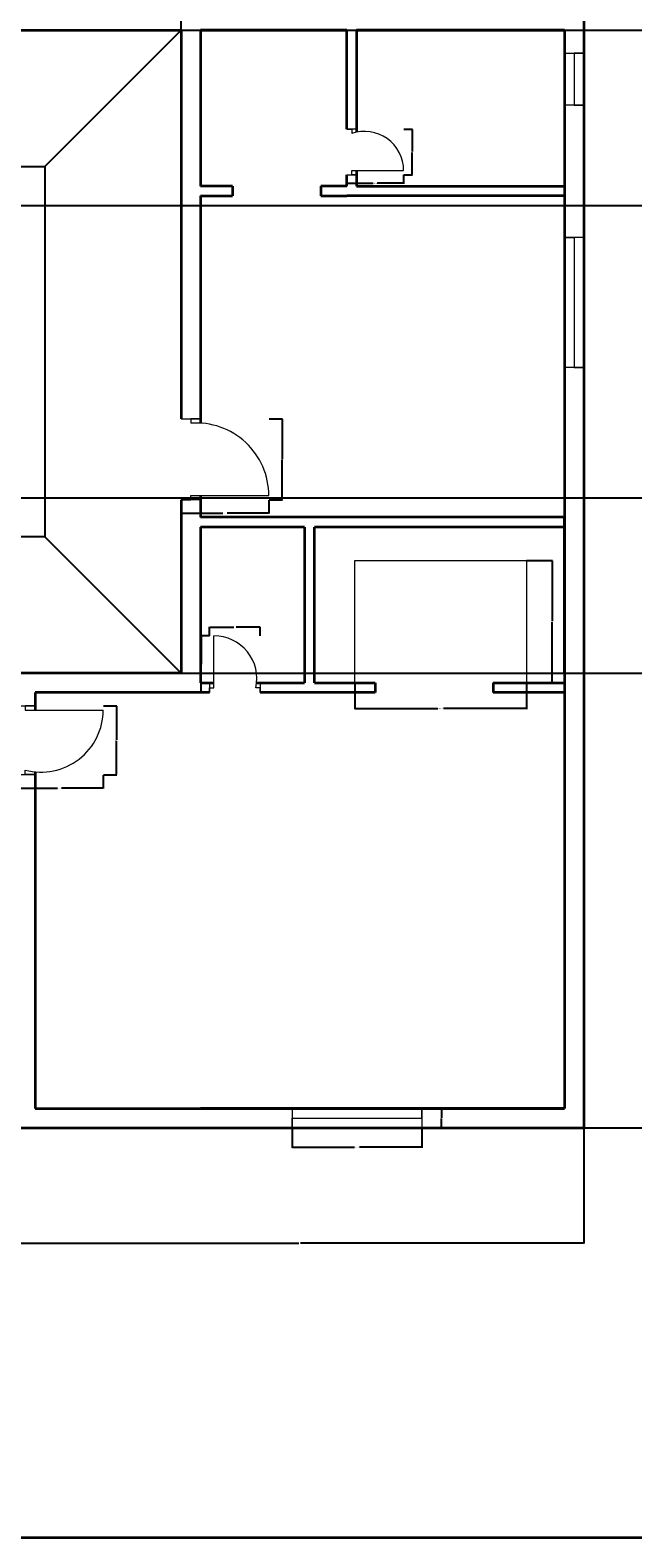
# Model space of a CAD drawing. Units: inches. Extents: x 2185 to 4426, y 1138 to 3073.
# Tile 10 of 14: x 3677 to 3955, y 1138 to 1834. Entities that reach past the tile are written whole.
import ezdxf

# ---------------------------------------------------------------- set-up
doc = ezdxf.new("R2010")
doc.units = ezdxf.units.IN
for name, color, linetype, lineweight in [('A-ANNO-DIMS', 2, 'Continuous', 18), ('A-ANNO-TTLB', 7, 'Continuous', 35), ('A-DOOR', 3, 'Continuous', 18), ('A-FLOR-CASE', 32, 'Continuous', 18), ('A-FLOR-EDGE', 7, 'Continuous', 25), ('A-GLAZ', 4, 'Continuous', 18), ('A-WALL', 7, 'Continuous', 35)]:
    doc.layers.add(name, color=color, linetype=linetype, lineweight=lineweight)
doc.styles.get("Standard").update_dxf_attribs({"font": 'arial.ttf'})
doc.dimstyles.get("Standard").update_dxf_attribs({"dimtxt": 0.18, "dimasz": 0.18, "dimexe": 0.18, "dimexo": 0.0625, "dimgap": 0.09, "dimtad": 0, "dimtih": 1, "dimtoh": 1, "dimdec": 4, "dimzin": 0, "dimdsep": 46, "dimtxsty": 'Standard', "dimcen": 0.09, "dimadec": 0, "dimazin": 0, "dimtfac": 1, "dimtdec": 4, "dimtofl": 0, "dimtmove": 0, "dimatfit": 3, "dimfxl": 1, "dimtolj": 1, "dimtzin": 0, "dimarcsym": 0})

# ---------------------------------------------------------------- blocks, each defined once
blk = doc.blocks.new('DOOR-SGL-24-BATH-S')
for p, q in [((2, 2.25), (2, 26.25)), ((0, 4.5), (0, 0)), ((0, 0), (0, 2.25)), ((0, 2.25), (0, 2.25)), ((0, 2.25), (2, 2.25)), ((23.36, 2.25), (21.36, 2.25)), ((23.36, 4.5), (23.36, 4.5)), ((23.36, 4.5), (23.36, 0)), ((23.36, 0), (23.36, 2.25))]:
    blk.add_line(p, q)
blk.add_arc((2, 6.44), 19.81, 347.78651, 90)
blk = doc.blocks.new('DOOR-SGL-36-BED-SE')
for p, q in [((0, 37.45), (9, 37.45)), ((9, 37.45), (4.5, 37.45)), ((4.5, 37.45), (4.5, 35.45)), ((9, 0), (0, 0)), ((0, 0), (4.5, 0)), ((4.5, 0), (4.5, 2)), ((4.5, 2), (40.5, 2))]:
    blk.add_line(p, q)
blk.add_arc((6.96, 2), 33.54, 0, 94.21362)
blk = doc.blocks.new('DOOR-SGL-24-BATH-E')
for p, q in [((4.5, 21.05), (0, 21.05)), ((0, 21.05), (2.25, 21.05)), ((2.25, 21.05), (2.25, 19.05)), ((0, 0), (4.5, 0)), ((2.25, 0), (2.25, 2)), ((2.25, 2), (26.25, 2)), ((4.5, 0), (2.25, 0))]:
    blk.add_line(p, q)
blk.add_arc((8.19, 2), 18.06, 0, 109.21567)
blk = doc.blocks.new('DOOR-SGL-36-BED-S')
for p, q in [((0, 31.73), (9, 31.73)), ((9, 31.73), (4.5, 31.73)), ((4.5, 31.73), (4.5, 31.73)), ((4.5, 31.73), (4.5, 29.73)), ((4.5, 29.73), (40.5, 29.73)), ((0, 0), (9, 0)), ((4.5, 0), (4.5, 2)), ((9, 0), (4.5, 0))]:
    blk.add_line(p, q)
blk.add_arc((11.82, 29.73), 28.68, 255.21093, 0)
blk = doc.blocks.new('WIN-PLAN-24IN-03')
for p, q in [((0, 24), (9, 24)), ((9, 24), (4.5, 24)), ((4.5, 24), (4.5, 0)), ((9, 0), (0, 0)), ((4.5, 0), (9, 0))]:
    blk.add_line(p, q)
blk = doc.blocks.new('WIN-PLAN-60IN-01')
for p, q in [((0, 9), (0, 0)), ((60, 4.5), (60, 9)), ((60, 9), (60, 0)), ((0, 0), (0, 4.5)), ((0, 4.5), (0, 4.5)), ((0, 4.5), (60, 4.5))]:
    blk.add_line(p, q)
blk = doc.blocks.new('WARDROBE-U')
for p, q in [((0, 0), (0, 56.6)), ((0, 56.6), (79.32, 56.6)), ((79.32, 56.6), (79.32, 0))]:
    blk.add_line(p, q)
blk = doc.blocks.new('*D60')
at = {"layer": 'A-ANNO-DIMS', "color": 0, "lineweight": -2, "transparency": 16777216}
for p, q in [((3797.54, 1327.31), (3797.54, 1318.2)), ((3857.54, 1327.31), (3857.54, 1318.2)), ((3797.72, 1318.38), (3826.42, 1318.38)), ((3857.36, 1318.38), (3828.66, 1318.38))]:
    blk.add_line(p, q, dxfattribs=at)
at = {"layer": 'A-ANNO-DIMS', "color": 0, "transparency": 16777216}
for points in [[(3797.72, 1318.41), (3797.72, 1318.35), (3797.54, 1318.38)], [(3857.36, 1318.41), (3857.36, 1318.35), (3857.54, 1318.38)]]:
    blk.add_solid(points, dxfattribs=at)
at = {"layer": 'Defpoints', "color": 0, "transparency": 16777216}
for p in [(3797.54, 1327.38), (3857.54, 1327.38), (3857.54, 1318.38)]:
    blk.add_point(p, dxfattribs=at)
at = {"layer": 'A-ANNO-DIMS', "color": 0, "transparency": 16777216, "insert": (3827.54, 1318.38), "char_height": 0.18, "attachment_point": 5}
blk.add_mtext('\\A1;WINDOW 60 TYP.', dxfattribs=at)
blk = doc.blocks.new('*D61')
at = {"layer": 'A-ANNO-DIMS', "color": 0, "lineweight": -2, "transparency": 16777216}
for p, q in [((3857.6, 1336.38), (3866.72, 1336.38)), ((3866.54, 1336.2), (3866.54, 1332.06)), ((3866.54, 1327.56), (3866.54, 1331.7)), ((3857.6, 1327.38), (3866.72, 1327.38))]:
    blk.add_line(p, q, dxfattribs=at)
at = {"layer": 'A-ANNO-DIMS', "color": 0, "transparency": 16777216}
for points in [[(3866.51, 1336.2), (3866.57, 1336.2), (3866.54, 1336.38)], [(3866.51, 1327.56), (3866.57, 1327.56), (3866.54, 1327.38)]]:
    blk.add_solid(points, dxfattribs=at)
at = {"layer": 'Defpoints', "color": 0, "transparency": 16777216}
for p in [(3857.54, 1336.38), (3866.54, 1336.38), (3857.54, 1327.38)]:
    blk.add_point(p, dxfattribs=at)
at = {"layer": 'A-ANNO-DIMS', "color": 0, "transparency": 16777216, "insert": (3866.54, 1331.88), "char_height": 0.18, "attachment_point": 5}
blk.add_mtext('\\A1;9 TYP.', dxfattribs=at)
blk = doc.blocks.new('*D78')
at = {"layer": 'A-ANNO-DIMS', "color": 0, "lineweight": -2, "transparency": 16777216}
for p, q in [((3759.43, 1554.63), (3755.38, 1554.63)), ((3755.56, 1554.45), (3755.56, 1541.69)), ((3755.56, 1528.56), (3755.56, 1541.32)), ((3759.43, 1528.38), (3755.38, 1528.38))]:
    blk.add_line(p, q, dxfattribs=at)
at = {"layer": 'A-ANNO-DIMS', "color": 0, "transparency": 16777216}
for points in [[(3755.53, 1554.45), (3755.59, 1554.45), (3755.56, 1554.63)], [(3755.53, 1528.56), (3755.59, 1528.56), (3755.56, 1528.38)]]:
    blk.add_solid(points, dxfattribs=at)
at = {"layer": 'Defpoints', "color": 0, "transparency": 16777216}
for p in [(3755.56, 1554.63), (3759.5, 1554.63), (3759.5, 1528.38)]:
    blk.add_point(p, dxfattribs=at)
at = {"layer": 'A-ANNO-DIMS', "color": 0, "transparency": 16777216, "insert": (3755.56, 1541.5), "char_height": 0.18, "attachment_point": 5}
blk.add_mtext('\\A1;DOOR 26 TYP.', dxfattribs=at)
blk = doc.blocks.new('*D79')
at = {"layer": 'A-ANNO-DIMS', "color": 0, "lineweight": -2, "transparency": 16777216}
for p, q in [((3759.5, 1554.69), (3759.5, 1558.74)), ((3759.68, 1558.56), (3770.65, 1558.56)), ((3782.68, 1558.56), (3771.71, 1558.56)), ((3782.86, 1554.69), (3782.86, 1558.74))]:
    blk.add_line(p, q, dxfattribs=at)
at = {"layer": 'A-ANNO-DIMS', "color": 0, "transparency": 16777216}
for points in [[(3759.68, 1558.59), (3759.68, 1558.53), (3759.5, 1558.56)], [(3782.68, 1558.59), (3782.68, 1558.53), (3782.86, 1558.56)]]:
    blk.add_solid(points, dxfattribs=at)
at = {"layer": 'Defpoints', "color": 0, "transparency": 16777216}
for p in [(3759.5, 1554.63), (3782.86, 1558.56), (3782.86, 1554.63)]:
    blk.add_point(p, dxfattribs=at)
at = {"layer": 'A-ANNO-DIMS', "color": 0, "transparency": 16777216, "insert": (3771.18, 1558.56), "char_height": 0.18, "attachment_point": 5}
blk.add_mtext('\\A1;23 TYP.', dxfattribs=at)
blk = doc.blocks.new('*D82')
at = {"layer": 'A-ANNO-DIMS', "color": 0, "lineweight": -2, "transparency": 16777216}
for p, q in [((3746.35, 1617.31), (3746.35, 1611.12)), ((3786.85, 1617.31), (3786.85, 1611.12)), ((3746.53, 1611.3), (3765.66, 1611.3)), ((3786.67, 1611.3), (3767.53, 1611.3))]:
    blk.add_line(p, q, dxfattribs=at)
at = {"layer": 'A-ANNO-DIMS', "color": 0, "transparency": 16777216}
for points in [[(3746.53, 1611.33), (3746.53, 1611.27), (3746.35, 1611.3)], [(3786.67, 1611.33), (3786.67, 1611.27), (3786.85, 1611.3)]]:
    blk.add_solid(points, dxfattribs=at)
at = {"layer": 'Defpoints', "color": 0, "transparency": 16777216}
for p in [(3746.35, 1617.38), (3786.85, 1617.38), (3786.85, 1611.3)]:
    blk.add_point(p, dxfattribs=at)
at = {"layer": 'A-ANNO-DIMS', "color": 0, "transparency": 16777216, "insert": (3766.6, 1611.3), "char_height": 0.18, "attachment_point": 5}
blk.add_mtext('\\A1;DOOR 41 TYP.', dxfattribs=at)
blk = doc.blocks.new('*D83')
at = {"layer": 'A-ANNO-DIMS', "color": 0, "lineweight": -2, "transparency": 16777216}
for p, q in [((3786.91, 1654.82), (3793.1, 1654.82)), ((3792.92, 1654.64), (3792.92, 1636.28)), ((3792.92, 1617.56), (3792.92, 1635.92)), ((3786.91, 1617.38), (3793.1, 1617.38))]:
    blk.add_line(p, q, dxfattribs=at)
at = {"layer": 'A-ANNO-DIMS', "color": 0, "transparency": 16777216}
for points in [[(3792.89, 1654.64), (3792.95, 1654.64), (3792.92, 1654.82)], [(3792.89, 1617.56), (3792.95, 1617.56), (3792.92, 1617.38)]]:
    blk.add_solid(points, dxfattribs=at)
at = {"layer": 'Defpoints', "color": 0, "transparency": 16777216}
for p in [(3786.85, 1654.82), (3792.92, 1654.82), (3786.85, 1617.38)]:
    blk.add_point(p, dxfattribs=at)
at = {"layer": 'A-ANNO-DIMS', "color": 0, "transparency": 16777216, "insert": (3792.92, 1636.1), "char_height": 0.18, "attachment_point": 5}
blk.add_mtext('\\A1;37 TYP.', dxfattribs=at)
blk = doc.blocks.new('*D84')
at = {"layer": 'A-ANNO-DIMS', "color": 0, "lineweight": -2, "transparency": 16777216}
for p, q in [((3822.85, 1767.5), (3822.85, 1763.45)), ((3823.03, 1763.63), (3835.04, 1763.63)), ((3848.92, 1763.63), (3836.91, 1763.63)), ((3849.1, 1767.5), (3849.1, 1763.45))]:
    blk.add_line(p, q, dxfattribs=at)
at = {"layer": 'A-ANNO-DIMS', "color": 0, "transparency": 16777216}
for points in [[(3823.03, 1763.66), (3823.03, 1763.6), (3822.85, 1763.63)], [(3848.92, 1763.66), (3848.92, 1763.6), (3849.1, 1763.63)]]:
    blk.add_solid(points, dxfattribs=at)
at = {"layer": 'Defpoints', "color": 0, "transparency": 16777216}
for p in [(3822.85, 1767.56), (3849.1, 1767.56), (3849.1, 1763.63)]:
    blk.add_point(p, dxfattribs=at)
at = {"layer": 'A-ANNO-DIMS', "color": 0, "transparency": 16777216, "insert": (3835.97, 1763.63), "char_height": 0.18, "attachment_point": 5}
blk.add_mtext('\\A1;DOOR 26 TYP.', dxfattribs=at)
blk = doc.blocks.new('*D85')
at = {"layer": 'A-ANNO-DIMS', "color": 0, "lineweight": -2, "transparency": 16777216}
for p, q in [((3849.16, 1788.61), (3853.22, 1788.61)), ((3853.04, 1788.43), (3853.04, 1778.27)), ((3853.04, 1767.74), (3853.04, 1777.91)), ((3849.16, 1767.56), (3853.22, 1767.56))]:
    blk.add_line(p, q, dxfattribs=at)
at = {"layer": 'A-ANNO-DIMS', "color": 0, "transparency": 16777216}
for points in [[(3853.01, 1788.43), (3853.07, 1788.43), (3853.04, 1788.61)], [(3853.01, 1767.74), (3853.07, 1767.74), (3853.04, 1767.56)]]:
    blk.add_solid(points, dxfattribs=at)
at = {"layer": 'Defpoints', "color": 0, "transparency": 16777216}
for p in [(3849.1, 1788.61), (3853.04, 1788.61), (3849.1, 1767.56)]:
    blk.add_point(p, dxfattribs=at)
at = {"layer": 'A-ANNO-DIMS', "color": 0, "transparency": 16777216, "insert": (3853.04, 1778.09), "char_height": 0.18, "attachment_point": 5}
blk.add_mtext('\\A1;21 TYP.', dxfattribs=at)
blk = doc.blocks.new('*D90')
at = {"layer": 'A-ANNO-DIMS', "color": 0, "lineweight": -2, "transparency": 16777216}
for p, q in [((3669.85, 1490.29), (3669.85, 1484.1)), ((3710.35, 1490.29), (3710.35, 1484.1)), ((3670.03, 1484.28), (3689.16, 1484.28)), ((3710.17, 1484.28), (3691.03, 1484.28))]:
    blk.add_line(p, q, dxfattribs=at)
at = {"layer": 'A-ANNO-DIMS', "color": 0, "transparency": 16777216}
for points in [[(3670.03, 1484.31), (3670.03, 1484.25), (3669.85, 1484.28)], [(3710.17, 1484.31), (3710.17, 1484.25), (3710.35, 1484.28)]]:
    blk.add_solid(points, dxfattribs=at)
at = {"layer": 'Defpoints', "color": 0, "transparency": 16777216}
for p in [(3669.85, 1490.36), (3710.35, 1490.36), (3710.35, 1484.28)]:
    blk.add_point(p, dxfattribs=at)
at = {"layer": 'A-ANNO-DIMS', "color": 0, "transparency": 16777216, "insert": (3690.1, 1484.28), "char_height": 0.18, "attachment_point": 5}
blk.add_mtext('\\A1;DOOR 41 TYP.', dxfattribs=at)
blk = doc.blocks.new('*D91')
at = {"layer": 'A-ANNO-DIMS', "color": 0, "lineweight": -2, "transparency": 16777216}
for p, q in [((3710.41, 1522.36), (3716.6, 1522.36)), ((3716.42, 1522.18), (3716.42, 1506.54)), ((3716.42, 1490.54), (3716.42, 1506.17)), ((3710.41, 1490.36), (3716.6, 1490.36))]:
    blk.add_line(p, q, dxfattribs=at)
at = {"layer": 'A-ANNO-DIMS', "color": 0, "transparency": 16777216}
for points in [[(3716.39, 1522.18), (3716.45, 1522.18), (3716.42, 1522.36)], [(3716.39, 1490.54), (3716.45, 1490.54), (3716.42, 1490.36)]]:
    blk.add_solid(points, dxfattribs=at)
at = {"layer": 'Defpoints', "color": 0, "transparency": 16777216}
for p in [(3710.35, 1522.36), (3716.42, 1522.36), (3710.35, 1490.36)]:
    blk.add_point(p, dxfattribs=at)
at = {"layer": 'A-ANNO-DIMS', "color": 0, "transparency": 16777216, "insert": (3716.42, 1506.36), "char_height": 0.18, "attachment_point": 5}
blk.add_mtext('\\A1;32 TYP.', dxfattribs=at)
blk = doc.blocks.new('*D122')
at = {"layer": 'A-ANNO-DIMS', "color": 0, "lineweight": -2, "transparency": 16777216}
for p, q in [((3826.51, 1532.81), (3826.51, 1520.8)), ((3905.83, 1532.81), (3905.83, 1520.8)), ((3826.69, 1520.98), (3864.86, 1520.98)), ((3905.65, 1520.98), (3867.48, 1520.98))]:
    blk.add_line(p, q, dxfattribs=at)
at = {"layer": 'A-ANNO-DIMS', "color": 0, "transparency": 16777216}
for points in [[(3826.69, 1521.01), (3826.69, 1520.95), (3826.51, 1520.98)], [(3905.65, 1521.01), (3905.65, 1520.95), (3905.83, 1520.98)]]:
    blk.add_solid(points, dxfattribs=at)
at = {"layer": 'Defpoints', "color": 0, "transparency": 16777216}
for p in [(3826.51, 1532.88), (3905.83, 1532.88), (3905.83, 1520.98)]:
    blk.add_point(p, dxfattribs=at)
at = {"layer": 'A-ANNO-DIMS', "color": 0, "transparency": 16777216, "insert": (3866.17, 1520.98), "char_height": 0.18, "attachment_point": 5}
blk.add_mtext('\\A1;WARDROBE 79 TYP.', dxfattribs=at)
blk = doc.blocks.new('*D123')
at = {"layer": 'A-ANNO-DIMS', "color": 0, "lineweight": -2, "transparency": 16777216}
for p, q in [((3905.89, 1589.48), (3917.91, 1589.48)), ((3917.73, 1589.3), (3917.73, 1561.36)), ((3917.73, 1533.06), (3917.73, 1561)), ((3905.89, 1532.88), (3917.91, 1532.88))]:
    blk.add_line(p, q, dxfattribs=at)
at = {"layer": 'A-ANNO-DIMS', "color": 0, "transparency": 16777216}
for points in [[(3917.7, 1589.3), (3917.76, 1589.3), (3917.73, 1589.48)], [(3917.7, 1533.06), (3917.76, 1533.06), (3917.73, 1532.88)]]:
    blk.add_solid(points, dxfattribs=at)
at = {"layer": 'Defpoints', "color": 0, "transparency": 16777216}
for p in [(3905.83, 1589.48), (3917.73, 1589.48), (3905.83, 1532.88)]:
    blk.add_point(p, dxfattribs=at)
at = {"layer": 'A-ANNO-DIMS', "color": 0, "transparency": 16777216, "insert": (3917.73, 1561.18), "char_height": 0.18, "attachment_point": 5}
blk.add_mtext('\\A1;57 TYP.', dxfattribs=at)
blk = doc.blocks.new('*D146')
at = {"layer": 'A-ANNO-DIMS', "color": 0, "lineweight": -2, "transparency": 16777216}
for p, q in [((3932.41, 2326.38), (4058.64, 2326.38)), ((4058.46, 2326.2), (4058.46, 1827.06)), ((4058.46, 1327.56), (4058.46, 1826.7)), ((3932.41, 1327.38), (4058.64, 1327.38))]:
    blk.add_line(p, q, dxfattribs=at)
at = {"layer": 'A-ANNO-DIMS', "color": 0, "transparency": 16777216}
for points in [[(4058.43, 2326.2), (4058.49, 2326.2), (4058.46, 2326.38)], [(4058.43, 1327.56), (4058.49, 1327.56), (4058.46, 1327.38)]]:
    blk.add_solid(points, dxfattribs=at)
at = {"layer": 'Defpoints', "color": 0, "transparency": 16777216}
for p in [(3932.35, 2326.38), (4058.46, 2326.38), (3932.35, 1327.38)]:
    blk.add_point(p, dxfattribs=at)
at = {"layer": 'A-ANNO-DIMS', "color": 0, "transparency": 16777216, "insert": (4058.46, 1826.88), "char_height": 0.18, "attachment_point": 5}
blk.add_mtext('\\A1;999', dxfattribs=at)
blk = doc.blocks.new('*D149')
at = {"layer": 'A-ANNO-DIMS', "color": 0, "lineweight": -2, "transparency": 16777216}
for p, q in [((3669.85, 1336.31), (3669.85, 1273.95)), ((3932.35, 1327.31), (3932.35, 1273.95)), ((3670.03, 1274.13), (3800.7, 1274.13)), ((3932.17, 1274.13), (3801.5, 1274.13))]:
    blk.add_line(p, q, dxfattribs=at)
at = {"layer": 'A-ANNO-DIMS', "color": 0, "transparency": 16777216}
for points in [[(3670.03, 1274.16), (3670.03, 1274.1), (3669.85, 1274.13)], [(3932.17, 1274.16), (3932.17, 1274.1), (3932.35, 1274.13)]]:
    blk.add_solid(points, dxfattribs=at)
at = {"layer": 'Defpoints', "color": 0, "transparency": 16777216}
for p in [(3669.85, 1336.38), (3932.35, 1327.38), (3932.35, 1274.13)]:
    blk.add_point(p, dxfattribs=at)
at = {"layer": 'A-ANNO-DIMS', "color": 0, "transparency": 16777216, "insert": (3801.1, 1274.13), "char_height": 0.18, "attachment_point": 5}
blk.add_mtext('\\A1;262.5', dxfattribs=at)
blk = doc.blocks.new('*D157')
at = {"layer": 'A-ANNO-DIMS', "color": 0, "lineweight": -2, "transparency": 16777216}
for p, q in [((3665.35, 1753.44), (3665.35, 2379.81)), ((3665.53, 2379.63), (3705.65, 2379.63)), ((3746.17, 2379.63), (3706.05, 2379.63)), ((3746.35, 1834.44), (3746.35, 2379.81))]:
    blk.add_line(p, q, dxfattribs=at)
at = {"layer": 'A-ANNO-DIMS', "color": 0, "transparency": 16777216}
for points in [[(3665.53, 2379.66), (3665.53, 2379.6), (3665.35, 2379.63)], [(3746.17, 2379.66), (3746.17, 2379.6), (3746.35, 2379.63)]]:
    blk.add_solid(points, dxfattribs=at)
at = {"layer": 'Defpoints', "color": 0, "transparency": 16777216}
for p in [(3746.35, 2379.63), (3746.35, 1834.38), (3665.35, 1753.38)]:
    blk.add_point(p, dxfattribs=at)
at = {"layer": 'A-ANNO-DIMS', "color": 0, "transparency": 16777216, "insert": (3705.85, 2379.63), "char_height": 0.18, "attachment_point": 5}
blk.add_mtext('\\A1;81', dxfattribs=at)
blk = doc.blocks.new('*D158')
at = {"layer": 'A-ANNO-DIMS', "color": 0, "lineweight": -2, "transparency": 16777216}
for p, q in [((3665.41, 1618.38), (4058.64, 1618.38)), ((4058.46, 1618.2), (4058.46, 1578.06)), ((4058.46, 1537.56), (4058.46, 1577.7)), ((3746.41, 1537.38), (4058.64, 1537.38))]:
    blk.add_line(p, q, dxfattribs=at)
at = {"layer": 'A-ANNO-DIMS', "color": 0, "transparency": 16777216}
for points in [[(4058.43, 1618.2), (4058.49, 1618.2), (4058.46, 1618.38)], [(4058.43, 1537.56), (4058.49, 1537.56), (4058.46, 1537.38)]]:
    blk.add_solid(points, dxfattribs=at)
at = {"layer": 'Defpoints', "color": 0, "transparency": 16777216}
for p in [(3665.35, 1618.38), (4058.46, 1618.38), (3746.35, 1537.38)]:
    blk.add_point(p, dxfattribs=at)
at = {"layer": 'A-ANNO-DIMS', "color": 0, "transparency": 16777216, "insert": (4058.46, 1577.88), "char_height": 0.18, "attachment_point": 5}
blk.add_mtext('\\A1;81', dxfattribs=at)
blk = doc.blocks.new('*D159')
at = {"layer": 'A-ANNO-DIMS', "color": 0, "lineweight": -2, "transparency": 16777216}
for p, q in [((3665.41, 1753.38), (4058.64, 1753.38)), ((4058.46, 1753.2), (4058.46, 1686.06)), ((4058.46, 1618.56), (4058.46, 1685.69)), ((3665.41, 1618.38), (4058.64, 1618.38))]:
    blk.add_line(p, q, dxfattribs=at)
at = {"layer": 'A-ANNO-DIMS', "color": 0, "transparency": 16777216}
for points in [[(4058.43, 1753.2), (4058.49, 1753.2), (4058.46, 1753.38)], [(4058.43, 1618.56), (4058.49, 1618.56), (4058.46, 1618.38)]]:
    blk.add_solid(points, dxfattribs=at)
at = {"layer": 'Defpoints', "color": 0, "transparency": 16777216}
for p in [(3665.35, 1753.38), (4058.46, 1753.38), (3665.35, 1618.38)]:
    blk.add_point(p, dxfattribs=at)
at = {"layer": 'A-ANNO-DIMS', "color": 0, "transparency": 16777216, "insert": (4058.46, 1685.88), "char_height": 0.18, "attachment_point": 5}
blk.add_mtext('\\A1;135', dxfattribs=at)
blk = doc.blocks.new('*D160')
at = {"layer": 'A-ANNO-DIMS', "color": 0, "lineweight": -2, "transparency": 16777216}
for p, q in [((3746.41, 1834.38), (4058.64, 1834.38)), ((4058.46, 1834.2), (4058.46, 1794.06)), ((4058.46, 1753.56), (4058.46, 1793.7)), ((3665.41, 1753.38), (4058.64, 1753.38))]:
    blk.add_line(p, q, dxfattribs=at)
at = {"layer": 'A-ANNO-DIMS', "color": 0, "transparency": 16777216}
for points in [[(4058.43, 1834.2), (4058.49, 1834.2), (4058.46, 1834.38)], [(4058.43, 1753.56), (4058.49, 1753.56), (4058.46, 1753.38)]]:
    blk.add_solid(points, dxfattribs=at)
at = {"layer": 'Defpoints', "color": 0, "transparency": 16777216}
for p in [(3746.35, 1834.38), (4058.46, 1834.38), (3665.35, 1753.38)]:
    blk.add_point(p, dxfattribs=at)
at = {"layer": 'A-ANNO-DIMS', "color": 0, "transparency": 16777216, "insert": (4058.46, 1793.88), "char_height": 0.18, "attachment_point": 5}
blk.add_mtext('\\A1;81', dxfattribs=at)

msp = doc.modelspace()

# ---------------------------------------------------------------- linework, layer by layer
at = {"layer": 'A-ANNO-TTLB'}
msp.add_lwpolyline([(2184.741, 3073.364), (4426.252, 3073.364), (4426.252, 1137.99), (2184.741, 1137.99)], close=True, dxfattribs=at)
at = {"layer": 'A-FLOR-EDGE'}
for p, q in [((3683.349, 1771.377), (3746.349, 1834.377)), ((3683.349, 1771.377), (3746.349, 1834.377)), ((3683.349, 1771.377), (3683.349, 1771.377)), ((3683.349, 1771.377), (3683.349, 1771.377)), ((3683.349, 1600.377), (3746.349, 1537.377)), ((3683.349, 1600.377), (3746.349, 1537.377))]:
    msp.add_line(p, q, dxfattribs=at)
msp.add_lwpolyline([(3411.807, 1771.377), (3683.349, 1771.377), (3683.349, 1600.377), (3411.807, 1600.377)], close=True, dxfattribs=at)
msp.add_lwpolyline([(3411.807, 1771.377), (3683.349, 1771.377), (3683.349, 1600.377), (3411.807, 1600.377)], close=True, dxfattribs=at)
at = {"layer": 'A-WALL'}
for p, q in [((3932.349, 2326.377), (3932.349, 1327.377)), ((3932.349, 2326.377), (3932.349, 1327.377)), ((3553.486, 1834.377), (3678.849, 1834.377)), ((3553.486, 1834.377), (3678.849, 1834.377)), ((3678.849, 1834.377), (3746.349, 1834.377)), ((3678.849, 1834.377), (3746.349, 1834.377)), ((3746.349, 1834.377), (3746.349, 1654.82)), ((3746.349, 1834.377), (3746.349, 1654.82)), ((3755.349, 1834.377), (3822.849, 1834.377)), ((3822.849, 1834.377), (3755.349, 1834.377)), ((3755.349, 1834.377), (3755.349, 1762.377)), ((3755.349, 1834.377), (3822.849, 1834.377)), ((3822.849, 1834.377), (3755.349, 1834.377)), ((3755.349, 1834.377), (3755.349, 1762.377)), ((3822.849, 1788.614), (3822.849, 1834.377)), ((3822.849, 1788.614), (3822.849, 1834.377)), ((3827.349, 1834.377), (3923.349, 1834.377)), ((3923.349, 1834.377), (3827.349, 1834.377)), ((3827.349, 1834.377), (3827.349, 1787.239)), ((3923.349, 1834.377), (3827.349, 1834.377)), ((3827.349, 1834.377), (3923.349, 1834.377)), ((3923.349, 1834.377), (3827.349, 1834.377)), ((3827.349, 1834.377), (3827.349, 1787.239)), ((3923.349, 1834.377), (3827.349, 1834.377)), ((3923.349, 1834.377), (3923.349, 1336.377)), ((3923.349, 1834.377), (3923.349, 1336.377)), ((3827.349, 1769.563), (3827.349, 1762.377)), ((3827.349, 1769.563), (3827.349, 1762.377)), ((3770.109, 1762.377), (3755.349, 1762.377)), ((3770.109, 1762.377), (3755.349, 1762.377)), ((3770.109, 1762.377), (3770.109, 1757.877)), ((3770.109, 1762.377), (3770.109, 1757.877)), ((3822.849, 1762.377), (3810.868, 1762.377)), ((3810.868, 1762.377), (3810.868, 1757.877)), ((3822.849, 1762.377), (3810.868, 1762.377)), ((3810.868, 1762.377), (3810.868, 1757.877)), ((3822.849, 1762.377), (3822.849, 1767.563)), ((3822.849, 1762.377), (3822.849, 1767.563)), ((3827.349, 1762.377), (3923.349, 1762.377)), ((3827.349, 1762.377), (3923.349, 1762.377)), ((3923.349, 1762.377), (3923.349, 1757.877)), ((3923.349, 1762.377), (3923.349, 1757.877)), ((3755.349, 1757.877), (3755.349, 1652.849)), ((3755.349, 1757.877), (3770.109, 1757.877)), ((3755.349, 1757.877), (3755.349, 1652.849)), ((3755.349, 1757.877), (3770.109, 1757.877)), ((3810.868, 1757.877), (3822.849, 1757.877)), ((3810.868, 1757.877), (3822.849, 1757.877)), ((3827.349, 1757.877), (3822.849, 1757.877)), ((3827.349, 1757.877), (3822.849, 1757.877)), ((3923.349, 1757.877), (3827.349, 1757.877)), ((3923.349, 1757.877), (3827.349, 1757.877)), ((3746.349, 1617.375), (3746.349, 1537.377)), ((3746.349, 1617.375), (3746.349, 1537.377)), ((3755.349, 1619.375), (3755.349, 1609.377)), ((3755.349, 1619.375), (3755.349, 1609.377)), ((3923.349, 1609.377), (3755.349, 1609.377)), ((3923.349, 1609.377), (3755.349, 1609.377)), ((3827.349, 1609.377), (3803.349, 1609.377)), ((3827.349, 1609.377), (3803.349, 1609.377)), ((3923.349, 1609.377), (3827.349, 1609.377)), ((3923.349, 1609.377), (3827.349, 1609.377)), ((3923.349, 1537.377), (3923.349, 1609.377)), ((3923.349, 1537.377), (3923.349, 1609.377)), ((3755.349, 1604.877), (3755.349, 1537.377)), ((3803.349, 1604.877), (3755.349, 1604.877)), ((3755.349, 1604.877), (3755.349, 1537.377)), ((3803.349, 1604.877), (3755.349, 1604.877)), ((3803.349, 1604.877), (3803.349, 1532.877)), ((3803.349, 1604.877), (3803.349, 1532.877)), ((3923.349, 1604.877), (3807.849, 1604.877)), ((3807.849, 1532.877), (3807.849, 1604.877)), ((3923.349, 1604.877), (3807.849, 1604.877)), ((3807.849, 1532.877), (3807.849, 1604.877)), ((3923.349, 1604.877), (3827.349, 1604.877)), ((3923.349, 1604.877), (3827.349, 1604.877)), ((3746.349, 1537.377), (3588.761, 1537.377)), ((3746.349, 1537.377), (3588.761, 1537.377)), ((3755.349, 1537.377), (3755.349, 1532.877)), ((3755.349, 1537.377), (3755.349, 1532.877)), ((3755.349, 1532.877), (3761.495, 1532.877)), ((3755.349, 1532.877), (3761.495, 1532.877)), ((3781.209, 1532.877), (3803.349, 1532.877)), ((3781.209, 1532.877), (3803.349, 1532.877)), ((3807.849, 1532.877), (3835.974, 1532.877)), ((3807.849, 1532.877), (3835.974, 1532.877)), ((3835.974, 1532.877), (3835.974, 1528.377)), ((3835.974, 1532.877), (3835.974, 1528.377)), ((3890.451, 1532.877), (3923.349, 1532.877)), ((3890.451, 1532.877), (3890.451, 1528.377)), ((3890.451, 1532.877), (3923.349, 1532.877)), ((3890.451, 1532.877), (3890.451, 1528.377)), ((3759.495, 1528.377), (3678.849, 1528.377)), ((3678.849, 1528.377), (3678.849, 1520.356)), ((3759.495, 1528.377), (3678.849, 1528.377)), ((3678.849, 1528.377), (3678.849, 1520.356)), ((3755.349, 1528.377), (3750.849, 1528.377)), ((3755.349, 1528.377), (3750.849, 1528.377)), ((3835.974, 1528.377), (3782.856, 1528.377)), ((3835.974, 1528.377), (3782.856, 1528.377)), ((3923.349, 1528.377), (3890.451, 1528.377)), ((3923.349, 1528.377), (3890.451, 1528.377)), ((3678.849, 1491.816), (3678.849, 1336.377)), ((3678.849, 1491.816), (3678.849, 1336.377)), ((3678.849, 1336.377), (3923.349, 1336.377)), ((3678.849, 1336.377), (3923.349, 1336.377)), ((3923.349, 1336.377), (3755.349, 1336.377)), ((3923.349, 1336.377), (3755.349, 1336.377)), ((3553.486, 1327.377), (3932.349, 1327.377)), ((3553.486, 1327.377), (3932.349, 1327.377))]:
    msp.add_line(p, q, dxfattribs=at)

# ---------------------------------------------------------------- block references
at = {"layer": 'A-DOOR'}
for name, p in [('DOOR-SGL-24-BATH-E', (3822.849, 1767.563)), ('DOOR-SGL-24-BATH-E', (3822.849, 1767.563)), ('DOOR-SGL-36-BED-SE', (3746.349, 1617.375)), ('DOOR-SGL-36-BED-SE', (3746.349, 1617.375)), ('DOOR-SGL-24-BATH-S', (3759.495, 1528.377)), ('DOOR-SGL-24-BATH-S', (3759.495, 1528.377)), ('DOOR-SGL-36-BED-S', (3669.849, 1490.627)), ('DOOR-SGL-36-BED-S', (3669.849, 1490.627))]:
    msp.add_blockref(name, p, dxfattribs=at)
at = {"layer": 'A-FLOR-CASE'}
msp.add_blockref('WARDROBE-U', (3826.507, 1532.877), dxfattribs=at)
msp.add_blockref('WARDROBE-U', (3826.507, 1532.877), dxfattribs=at)
at = {"layer": 'A-GLAZ'}
for name, p in [('WIN-PLAN-24IN-03', (3923.349, 1799.715)), ('WIN-PLAN-24IN-03', (3923.349, 1799.715)), ('WIN-PLAN-60IN-01', (3797.541, 1327.377)), ('WIN-PLAN-60IN-01', (3797.541, 1327.377))]:
    msp.add_blockref(name, p, dxfattribs=at)
at = {"layer": 'A-GLAZ', "rotation": 269.9999999999992}
msp.add_blockref('WIN-PLAN-60IN-01', (3923.349, 1738.584), dxfattribs=at)
msp.add_blockref('WIN-PLAN-60IN-01', (3923.349, 1738.584), dxfattribs=at)

# ---------------------------------------------------------------- dimensions: what is measured, and where the dimension line sits
at = {"layer": 'A-ANNO-DIMS'}
for base, p1, p2, override, picture, middle in [((3746.349, 2379.627), (3665.349, 1753.377), (3746.349, 1834.377), {"dimdec": 0, "dimlfac": 1, "dimrnd": 0, "dimzin": 0, "dimdsep": 46, "dimlunit": 2}, '*D157', (3705.849, 2379.627)), ((3932.349, 1274.127), (3669.849, 1336.377), (3932.349, 1327.377), {"dimdec": 1, "dimlfac": 1, "dimrnd": 0, "dimzin": 0, "dimdsep": 46, "dimlunit": 2}, '*D149', (3801.099, 1274.127))]:
    dim = msp.add_linear_dim(base=base, p1=p1, p2=p2, dimstyle='Standard', override=override, dxfattribs=at)
    dim.commit()
    dim.dimension.update_dxf_attribs({"geometry": picture, "text_midpoint": middle})
for base, p1, p2, picture, middle in [((4058.46, 2326.377), (3932.349, 1327.377), (3932.349, 2326.377), '*D146', (4058.46, 1826.877)), ((4058.46, 1834.377), (3665.349, 1753.377), (3746.349, 1834.377), '*D160', (4058.46, 1793.877)), ((4058.46, 1753.377), (3665.349, 1618.377), (3665.349, 1753.377), '*D159', (4058.46, 1685.877)), ((4058.46, 1618.377), (3746.349, 1537.377), (3665.349, 1618.377), '*D158', (4058.46, 1577.877))]:
    dim = msp.add_linear_dim(base=base, p1=p1, p2=p2, angle=90, dimstyle='Standard', override={"dimdec": 0, "dimlfac": 1, "dimrnd": 0, "dimzin": 0, "dimdsep": 46, "dimlunit": 2}, dxfattribs=at)
    dim.commit()
    dim.dimension.update_dxf_attribs({"geometry": picture, "text_midpoint": middle})
for base, p1, p2, text, picture, middle in [((3853.037, 1788.614), (3849.099, 1767.563), (3849.099, 1788.614), '<> TYP.', '*D85', (3853.037, 1778.089)), ((3792.924, 1654.82), (3786.849, 1617.375), (3786.849, 1654.82), '<> TYP.', '*D83', (3792.924, 1636.098)), ((3917.73, 1589.48), (3905.831, 1532.877), (3905.831, 1589.48), '<> TYP.', '*D123', (3917.73, 1561.178)), ((3755.558, 1554.627), (3759.495, 1528.377), (3759.495, 1554.627), 'DOOR <> TYP.', '*D78', (3755.558, 1541.502)), ((3716.424, 1522.356), (3710.349, 1490.356), (3710.349, 1522.356), '<> TYP.', '*D91', (3716.424, 1506.356)), ((3866.54, 1336.377), (3857.54, 1327.377), (3857.54, 1336.377), '<> TYP.', '*D61', (3866.54, 1331.877))]:
    dim = msp.add_linear_dim(base=base, p1=p1, p2=p2, angle=90, text=text, dimstyle='Standard', override={"dimdec": 0, "dimlfac": 1, "dimrnd": 0, "dimzin": 0, "dimdsep": 46, "dimlunit": 2}, dxfattribs=at)
    dim.commit()
    dim.dimension.update_dxf_attribs({"geometry": picture, "text_midpoint": middle})
for base, p1, p2, text, picture, middle in [((3849.099, 1763.626), (3822.849, 1767.563), (3849.099, 1767.563), 'DOOR <> TYP.', '*D84', (3835.974, 1763.626)), ((3786.84919158, 1611.30013454), (3746.34919158, 1617.37513454), (3786.84919158, 1617.37513454), 'DOOR <> TYP.', '*D82', (3766.59919158, 1611.30013454)), ((3782.856, 1558.564), (3759.495, 1554.627), (3782.856, 1554.627), '<> TYP.', '*D79', (3771.175, 1558.564)), ((3905.831, 1520.978), (3826.507, 1532.877), (3905.831, 1532.877), 'WARDROBE <> TYP.', '*D122', (3866.169, 1520.978)), ((3710.34919158, 1484.281003331), (3669.84919158, 1490.356003331), (3710.34919158, 1490.356003331), 'DOOR <> TYP.', '*D90', (3690.09919158, 1484.281003331)), ((3857.54, 1318.377), (3797.54, 1327.377), (3857.54, 1327.377), 'WINDOW <> TYP.', '*D60', (3827.54, 1318.377))]:
    dim = msp.add_linear_dim(base=base, p1=p1, p2=p2, text=text, dimstyle='Standard', override={"dimdec": 0, "dimlfac": 1, "dimrnd": 0, "dimzin": 0, "dimdsep": 46, "dimlunit": 2}, dxfattribs=at)
    dim.commit()
    dim.dimension.update_dxf_attribs({"geometry": picture, "text_midpoint": middle})

doc.saveas('drawing.dxf')
